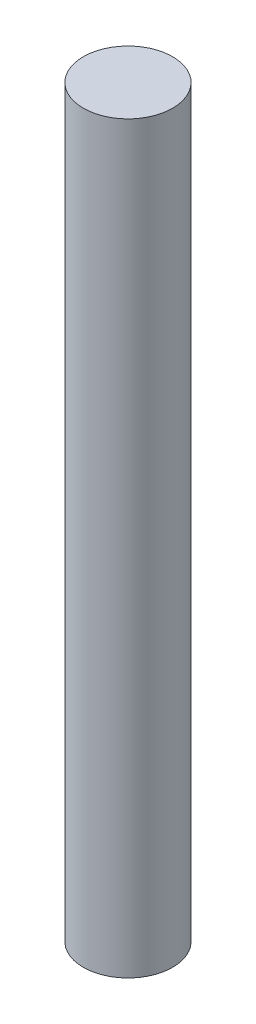
ISO-10303-21;
HEADER;
FILE_DESCRIPTION(('STEP AP214'),'2;1');
FILE_NAME('part.step','',(''),(''),'','','');
FILE_SCHEMA(('AUTOMOTIVE_DESIGN { 1 0 10303 214 1 1 1 1 }'));
ENDSEC;
DATA;
#1=APPLICATION_CONTEXT('core data for automotive mechanical design processes');
#2=APPLICATION_PROTOCOL_DEFINITION('international standard','automotive_design',2000,#1);
#3=PRODUCT_CONTEXT('',#1,'mechanical');
#4=PRODUCT('Part','Part','',(#3));
#5=PRODUCT_RELATED_PRODUCT_CATEGORY('part','',(#4));
#6=PRODUCT_DEFINITION_FORMATION('','',#4);
#7=PRODUCT_DEFINITION_CONTEXT('part definition',#1,'design');
#8=PRODUCT_DEFINITION('design','',#6,#7);
#9=PRODUCT_DEFINITION_SHAPE('','',#8);
#10=(LENGTH_UNIT() NAMED_UNIT(*) SI_UNIT(.MILLI.,.METRE.));
#11=(NAMED_UNIT(*) PLANE_ANGLE_UNIT() SI_UNIT($,.RADIAN.));
#12=(NAMED_UNIT(*) SI_UNIT($,.STERADIAN.) SOLID_ANGLE_UNIT());
#13=UNCERTAINTY_MEASURE_WITH_UNIT(LENGTH_MEASURE(1.E-05),#10,'distance_accuracy_value','');
#14=(GEOMETRIC_REPRESENTATION_CONTEXT(3) GLOBAL_UNCERTAINTY_ASSIGNED_CONTEXT((#13)) GLOBAL_UNIT_ASSIGNED_CONTEXT((#10,
#11,#12)) REPRESENTATION_CONTEXT('',''));
#15=CARTESIAN_POINT('',(0.,0.,0.));
#16=DIRECTION('',(0.,0.,1.));
#17=DIRECTION('',(1.,0.,0.));
#18=AXIS2_PLACEMENT_3D('',#15,#16,#17);
#19=CARTESIAN_POINT('',(0.,200.,0.));
#20=DIRECTION('',(0.,-1.,0.));
#21=DIRECTION('',(0.,0.,-1.));
#22=AXIS2_PLACEMENT_3D('',#19,#20,#21);
#23=CYLINDRICAL_SURFACE('',#22,12.);
#24=CARTESIAN_POINT('',(0.,200.,0.));
#25=DIRECTION('',(0.,1.,0.));
#26=DIRECTION('',(0.,0.,1.));
#27=AXIS2_PLACEMENT_3D('',#24,#25,#26);
#28=CIRCLE('',#27,12.);
#29=CARTESIAN_POINT('',(0.,200.,12.));
#30=VERTEX_POINT('',#29);
#31=EDGE_CURVE('E10',#30,#30,#28,.T.);
#32=ORIENTED_EDGE('',*,*,#31,.F.);
#33=EDGE_LOOP('',(#32));
#34=FACE_BOUND('',#33,.T.);
#35=CARTESIAN_POINT('',(0.,0.,0.));
#36=DIRECTION('',(0.,1.,0.));
#37=DIRECTION('',(0.,0.,1.));
#38=AXIS2_PLACEMENT_3D('',#35,#36,#37);
#39=CIRCLE('',#38,12.);
#40=CARTESIAN_POINT('',(0.,0.,12.));
#41=VERTEX_POINT('',#40);
#42=EDGE_CURVE('E37',#41,#41,#39,.T.);
#43=ORIENTED_EDGE('',*,*,#42,.T.);
#44=EDGE_LOOP('',(#43));
#45=FACE_BOUND('',#44,.T.);
#46=ADVANCED_FACE('F40',(#34,#45),#23,.T.);
#47=CARTESIAN_POINT('',(0.,200.,0.));
#48=DIRECTION('',(0.,1.,0.));
#49=DIRECTION('',(0.,0.,1.));
#50=AXIS2_PLACEMENT_3D('',#47,#48,#49);
#51=PLANE('',#50);
#52=ORIENTED_EDGE('',*,*,#31,.T.);
#53=EDGE_LOOP('',(#52));
#54=FACE_BOUND('',#53,.T.);
#55=ADVANCED_FACE('F55',(#54),#51,.T.);
#56=CARTESIAN_POINT('',(0.,0.,0.));
#57=DIRECTION('',(0.,1.,0.));
#58=DIRECTION('',(0.,0.,1.));
#59=AXIS2_PLACEMENT_3D('',#56,#57,#58);
#60=PLANE('',#59);
#61=ORIENTED_EDGE('',*,*,#42,.F.);
#62=EDGE_LOOP('',(#61));
#63=FACE_BOUND('',#62,.T.);
#64=ADVANCED_FACE('F49',(#63),#60,.F.);
#65=CLOSED_SHELL('',(#46,#55,#64));
#66=MANIFOLD_SOLID_BREP('B2',#65);
#67=ADVANCED_BREP_SHAPE_REPRESENTATION('',(#18,#66),#14);
#68=SHAPE_DEFINITION_REPRESENTATION(#9,#67);
ENDSEC;
END-ISO-10303-21;
